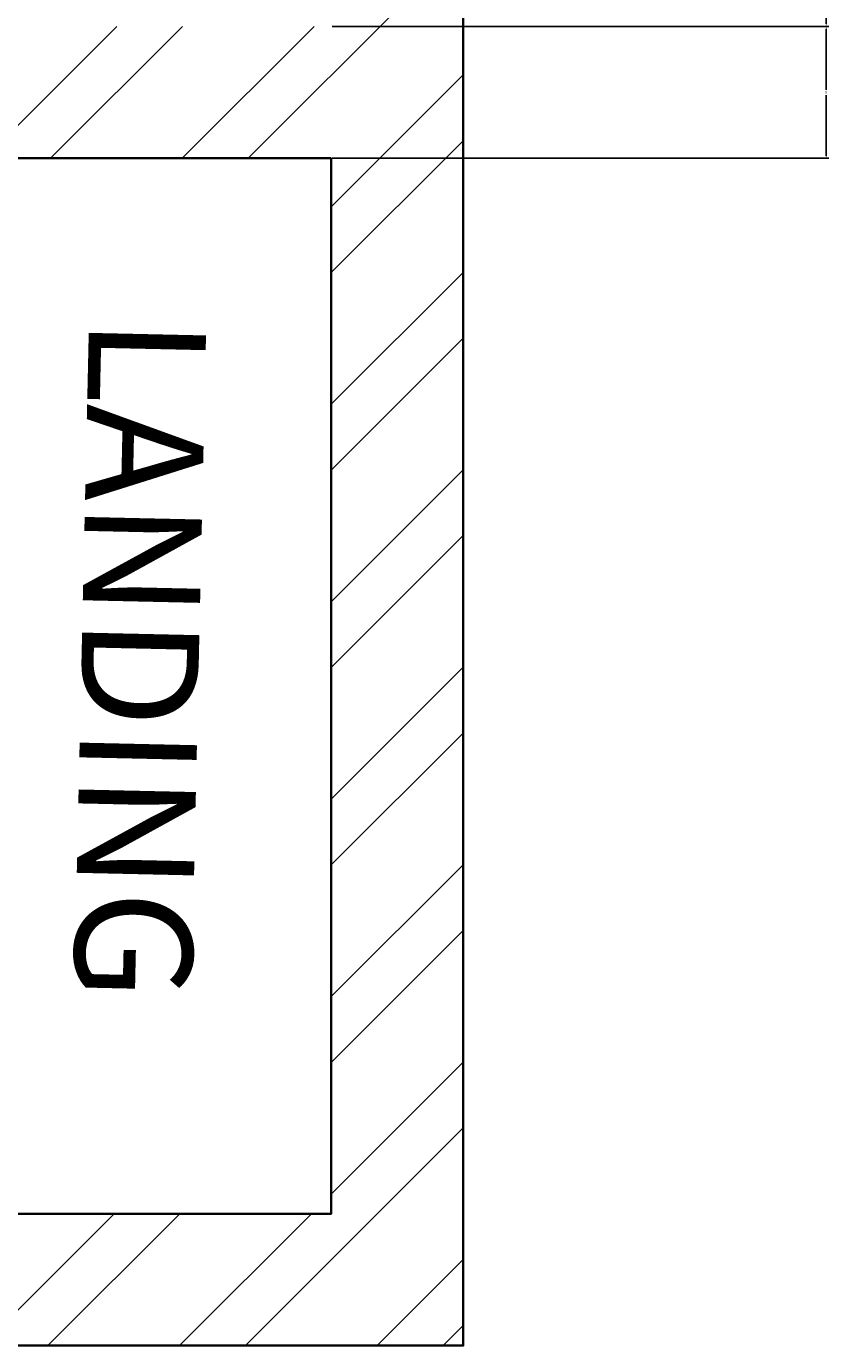
# Model space of a CAD drawing. Units: inches. Extents: x 2166 to 3588, y 1959 to 2628.
# Tile 11 of 13: x 3534 to 3588, y 2022 to 2112. Entities that reach past the tile are written whole.
import ezdxf

# ---------------------------------------------------------------- set-up
doc = ezdxf.new("R2010")
doc.units = ezdxf.units.IN
for name, color, linetype, lineweight in [('A-ANNO-DIMS', 2, 'Continuous', 18), ('A-AREA-IDEN', 170, 'Continuous', 18), ('A-WALL-PATT', 20, 'Continuous', 13), ('WALL', 40, 'Continuous', 35)]:
    doc.layers.add(name, color=color, linetype=linetype, lineweight=lineweight)
doc.styles.get("Standard").update_dxf_attribs({"font": 'arial.ttf'})
doc.dimstyles.get("Standard").update_dxf_attribs({"dimtxt": 0.18, "dimasz": 0.18, "dimexe": 0.18, "dimexo": 0.0625, "dimgap": 0.09, "dimtad": 0, "dimtih": 1, "dimtoh": 1, "dimdec": 4, "dimzin": 0, "dimdsep": 46, "dimtxsty": 'Standard', "dimcen": 0.09, "dimadec": 0, "dimazin": 0, "dimtfac": 1, "dimtdec": 4, "dimtofl": 0, "dimtmove": 0, "dimatfit": 3, "dimfxl": 1, "dimtolj": 1, "dimtzin": 0, "dimarcsym": 0})

# ---------------------------------------------------------------- blocks, each defined once
blk = doc.blocks.new('*D49')
at = {"layer": 'A-ANNO-DIMS', "color": 0, "lineweight": -2, "transparency": 16777216}
for p, q in [((3554.533, 2420.979), (3588.401, 2420.979)), ((3588.221, 2420.799), (3588.221, 2266.661)), ((3588.221, 2112.159), (3588.221, 2266.297)), ((3554.533, 2111.979), (3588.401, 2111.979))]:
    blk.add_line(p, q, dxfattribs=at)
at = {"layer": 'A-ANNO-DIMS', "color": 0, "transparency": 16777216}
for points in [[(3588.191, 2420.799), (3588.251, 2420.799), (3588.221, 2420.979)], [(3588.191, 2112.159), (3588.251, 2112.159), (3588.221, 2111.979)]]:
    blk.add_solid(points, dxfattribs=at)
at = {"layer": 'Defpoints', "color": 0, "transparency": 16777216}
for p in [(3554.471, 2420.979), (3588.221, 2420.979), (3554.471, 2111.979)]:
    blk.add_point(p, dxfattribs=at)
at = {"layer": 'A-ANNO-DIMS', "color": 0, "transparency": 16777216, "insert": (3588.221, 2266.479), "char_height": 0.18, "attachment_point": 5}
blk.add_mtext('\\A1;309', dxfattribs=at)
blk = doc.blocks.new('*D51')
at = {"layer": 'A-ANNO-DIMS', "color": 0, "lineweight": -2, "transparency": 16777216}
for p, q in [((3554.533, 2111.979), (3588.401, 2111.979)), ((3588.221, 2111.799), (3588.221, 2107.661)), ((3588.221, 2103.159), (3588.221, 2107.297)), ((3554.533, 2102.979), (3588.401, 2102.979))]:
    blk.add_line(p, q, dxfattribs=at)
at = {"layer": 'A-ANNO-DIMS', "color": 0, "transparency": 16777216}
for points in [[(3588.191, 2111.799), (3588.251, 2111.799), (3588.221, 2111.979)], [(3588.191, 2103.159), (3588.251, 2103.159), (3588.221, 2102.979)]]:
    blk.add_solid(points, dxfattribs=at)
at = {"layer": 'Defpoints', "color": 0, "transparency": 16777216}
for p in [(3554.471, 2111.979), (3588.221, 2111.979), (3554.471, 2102.979)]:
    blk.add_point(p, dxfattribs=at)
at = {"layer": 'A-ANNO-DIMS', "color": 0, "transparency": 16777216, "insert": (3588.221, 2107.479), "char_height": 0.18, "attachment_point": 5}
blk.add_mtext('\\A1;9', dxfattribs=at)

msp = doc.modelspace()

# ---------------------------------------------------------------- hatches: boundary and pattern name
at = {"layer": 'A-WALL-PATT'}
h = msp.add_hatch(dxfattribs=at)
h.set_pattern_fill('ANSI32', color=256)
h.paths.add_polyline_path([(3563.471, 2429.979), (3227.471, 2429.979), (3227.471, 2021.979), (3563.471, 2021.979)])
h.paths.add_polyline_path([(3236.471, 2420.979), (3554.471, 2420.979), (3554.471, 2111.979), (3236.471, 2111.979)], flags=16)
h.paths.add_polyline_path([(3236.471, 2102.979), (3554.471, 2102.979), (3554.471, 2030.979), (3236.471, 2030.979)], flags=16)
h.paths.add_polyline_path([(3518.471, 2085.283), (3518.471, 2067.979), (3458.471, 2067.979), (3458.471, 2085.283)], flags=0)
h.paths.add_polyline_path([(3434.656, 2082.283), (3442.194, 2082.283), (3442.194, 2087.514), (3434.656, 2087.514)], flags=8)
h.paths.add_polyline_path([(3522.671, 2094.512), (3521.752, 2052.984), (3545.541, 2052.457), (3546.46, 2093.986)], flags=8)

# ---------------------------------------------------------------- linework, layer by layer
at = {"layer": 'WALL'}
for q in [(3236.471, 2102.979), (3554.471, 2030.979)]:
    msp.add_line((3554.471, 2102.979), q, dxfattribs=at)
msp.add_lwpolyline([(3227.471, 2429.979), (3563.471, 2429.979), (3563.471, 2021.979), (3227.471, 2021.979)], close=True, dxfattribs=at)
msp.add_lwpolyline([(3554.471, 2102.979), (3554.471, 2030.979), (3236.471, 2030.979), (3236.471, 2102.979)], dxfattribs=at)

# ---------------------------------------------------------------- texts
at = {"layer": 'A-AREA-IDEN', "insert": (3545.955, 2091.996), "char_height": 8, "attachment_point": 1, "rotation": 268.73191}
msp.add_mtext_dynamic_manual_height_columns("{\\Fsuperos|c0;LANDING\\P   3'}", width=58.85395, gutter_width=12.5, heights=[0], dxfattribs=at)

# ---------------------------------------------------------------- dimensions: what is measured, and where the dimension line sits
at = {"layer": 'A-ANNO-DIMS'}
for base, p1, p2, picture, middle in [((3588.221, 2420.979), (3554.471, 2111.979), (3554.471, 2420.979), '*D49', (3588.221, 2266.479)), ((3588.221, 2111.979), (3554.471, 2102.979), (3554.471, 2111.979), '*D51', (3588.221, 2107.479))]:
    dim = msp.add_linear_dim(base=base, p1=p1, p2=p2, angle=90, dimstyle='Standard', override={"dimdec": 0, "dimlfac": 1, "dimrnd": 0, "dimzin": 0, "dimdsep": 46, "dimlunit": 2}, dxfattribs=at)
    dim.commit()
    dim.dimension.update_dxf_attribs({"geometry": picture, "text_midpoint": middle})

doc.saveas('drawing.dxf')
